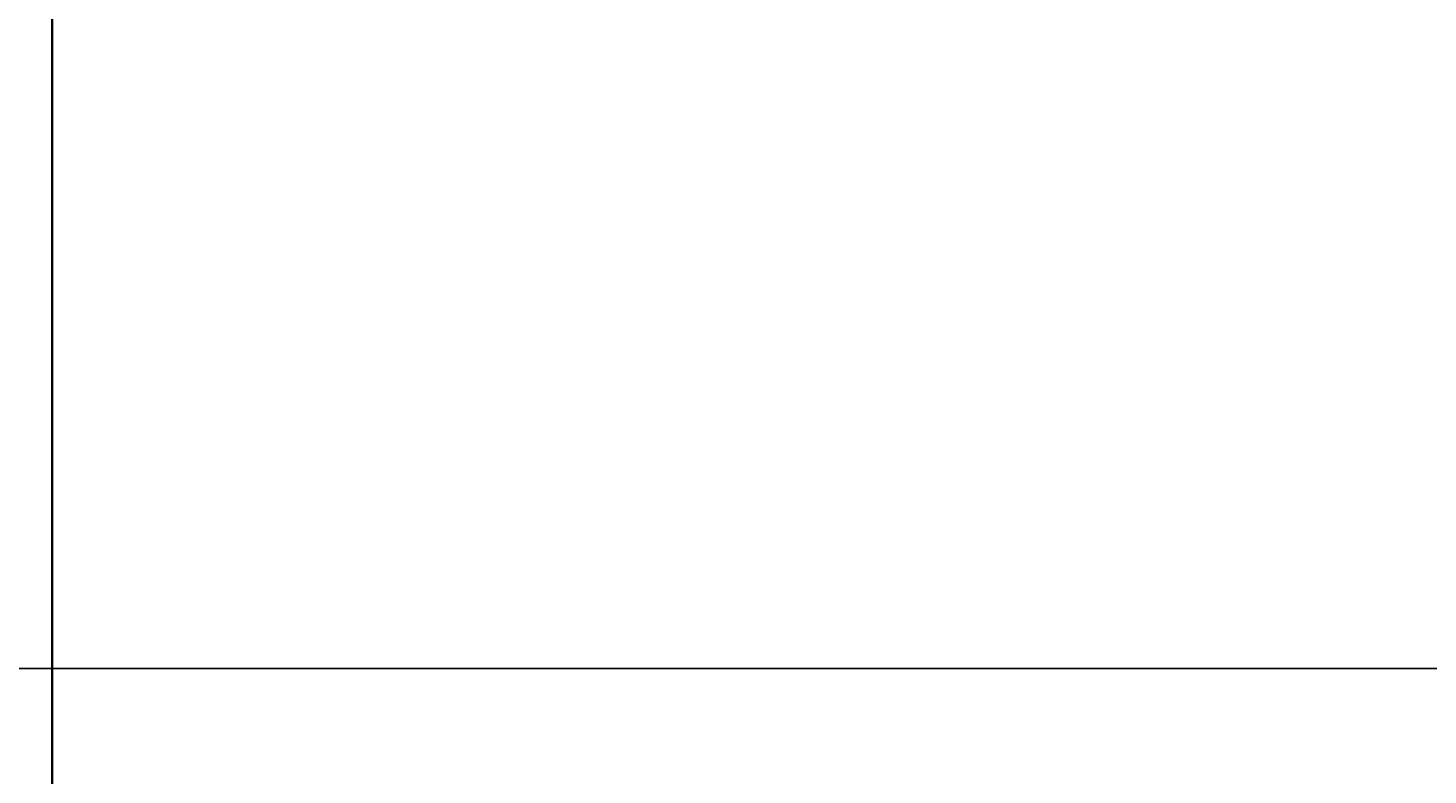
# Model space of a CAD drawing. Units: inches. Extents: x -61 to 1599, y -1316 to 257.
# Tile 184 of 204: x 998 to 1233, y -579 to -454. Entities that reach past the tile are written whole.
import ezdxf

# ---------------------------------------------------------------- set-up
doc = ezdxf.new("R2010")
doc.units = ezdxf.units.IN
doc.header["$MEASUREMENT"] = 0
doc.layers.add('A-ANNO-DIMS', color=2, linetype='Continuous', lineweight=18)
doc.layers.add('WALLS', color=4, linetype='Continuous', lineweight=35)
doc.styles.get("Standard").update_dxf_attribs({"font": 'arial.ttf'})
doc.dimstyles.get("Standard").update_dxf_attribs({"dimtxt": 0.18, "dimasz": 0.18, "dimexe": 0.18, "dimexo": 0.0625, "dimgap": 0.09, "dimtad": 0, "dimtih": 1, "dimtoh": 1, "dimdec": 0, "dimzin": 0, "dimdsep": 46, "dimlunit": 3, "dimtxsty": 'Standard', "dimcen": 0.09, "dimadec": 0, "dimazin": 0, "dimtfac": 1, "dimtdec": 0, "dimtofl": 0, "dimtmove": 0, "dimatfit": 3, "dimfxl": 1, "dimtolj": 1, "dimtzin": 0, "dimarcsym": 0})

# ---------------------------------------------------------------- blocks, each defined once
blk = doc.blocks.new('*D698')
at = {"layer": 'A-ANNO-DIMS', "color": 0, "lineweight": -2, "transparency": 16777216}
for p, q in [((644.77, -167.17), (1598.48, -167.17)), ((1598.3, -167.35), (1598.3, -363.99)), ((1598.3, -560.99), (1598.3, -364.35)), ((644.77, -561.17), (1598.48, -561.17))]:
    blk.add_line(p, q, dxfattribs=at)
at = {"layer": 'A-ANNO-DIMS', "color": 0, "transparency": 16777216}
for points in [[(1598.27, -167.35), (1598.33, -167.35), (1598.3, -167.17)], [(1598.27, -560.99), (1598.33, -560.99), (1598.3, -561.17)]]:
    blk.add_solid(points, dxfattribs=at)
at = {"layer": 'DEFPOINTS', "color": 0, "transparency": 16777216}
for p in [(644.7, -167.17), (1598.3, -167.17), (644.7, -561.17)]:
    blk.add_point(p, dxfattribs=at)
at = {"layer": 'A-ANNO-DIMS', "color": 0, "transparency": 16777216, "insert": (1598.3, -364.17), "char_height": 0.18, "attachment_point": 5}
blk.add_mtext('\\A1;394', dxfattribs=at)

msp = doc.modelspace()

# ---------------------------------------------------------------- linework, layer by layer
at = {"layer": 'WALLS'}
msp.add_line((1001.7028, -432.3229), (1001.7028, -741.169), dxfattribs=at)

# ---------------------------------------------------------------- dimensions: what is measured, and where the dimension line sits
at = {"layer": 'A-ANNO-DIMS'}
dim = msp.add_linear_dim(base=(1598.3028, -167.169), p1=(644.7028, -561.169), p2=(644.7028, -167.169), angle=90, dimstyle='Standard', override={"dimdec": 0, "dimlfac": 1, "dimrnd": 0, "dimzin": 0, "dimdsep": 46, "dimlunit": 2}, dxfattribs=at)
dim.commit()
dim.dimension.update_dxf_attribs({"geometry": '*D698', "text_midpoint": (1598.3028, -364.169)})

doc.saveas('drawing.dxf')
